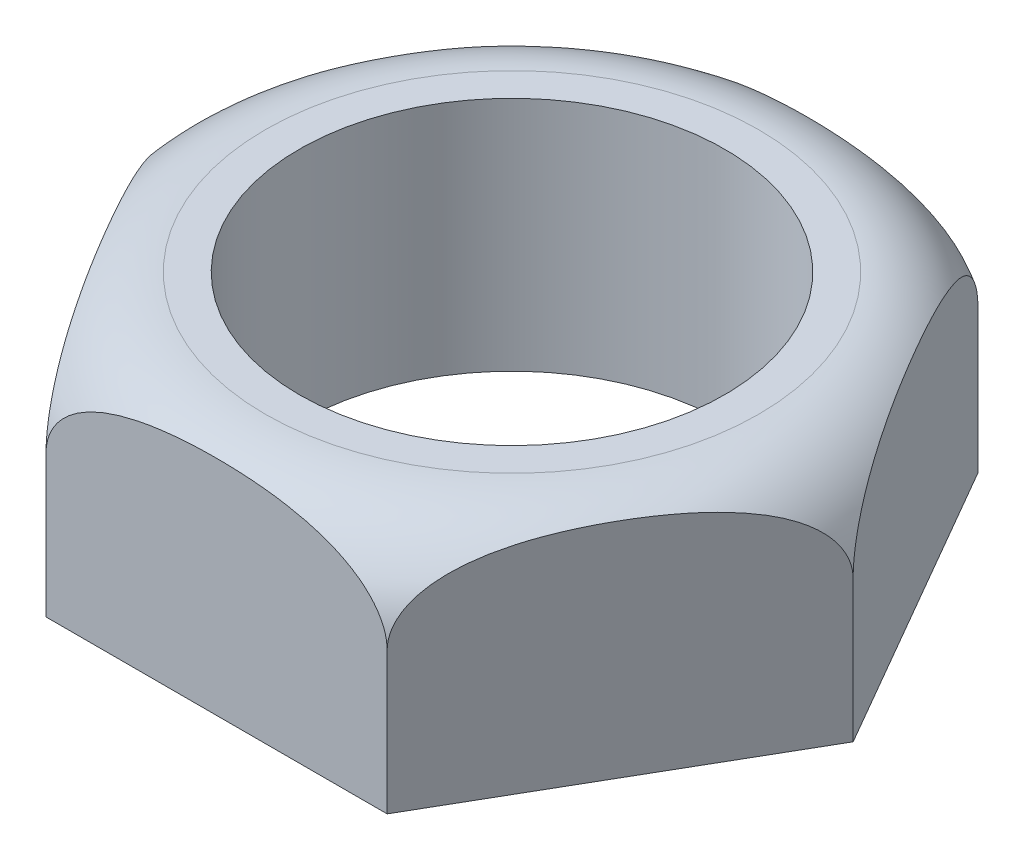
from build123d import *

# Parameters (mm, degrees)
HEX_PROFILE_SKETCH_R = 9
HEX_NUT_BODY_DEPTH   = 5


with BuildPart() as part:
    # Hex Profile Sketch → Hex Nut Body (new, symmetric)
    with BuildSketch(Plane(origin=(0, 0, 0), x_dir=(1, 0, 0), z_dir=(0, 1, 0))):
        Polygon((14.43375673, 0), (7.216878365, 12.5), (-7.216878365, 12.5), (-14.43375673, 0), (-7.216878365, -12.5), (7.216878365, -12.5), align=None)
        with Locations(Location((0, 0, 0), (0, 0, 270))):
            Circle(HEX_PROFILE_SKETCH_R, mode=Mode.SUBTRACT)
    extrude(amount=HEX_NUT_BODY_DEPTH, both=True)

    # Chamfer Profile Sketch → Nut Chamfer Cut (revolve, cut)
    with BuildSketch(Plane.XY, mode=Mode.PRIVATE) as nut_chamfer_cut_sk:
        with BuildLine():
            Line((10.43375673, 5), (14.43375673, 5))
            Line((14.43375673, 5), (14.43375673, 1))
            ThreePointArc((14.43375673, 1), (13.262183854, 3.828427125), (10.43375673, 5))
        make_face()
    revolve(nut_chamfer_cut_sk.sketch.rotate(Axis((0, 0, 0), (0, 1, 0)), 90), axis=Axis((0, 0, 0), (0, 1, 0)), mode=Mode.SUBTRACT)


solid = part.part
